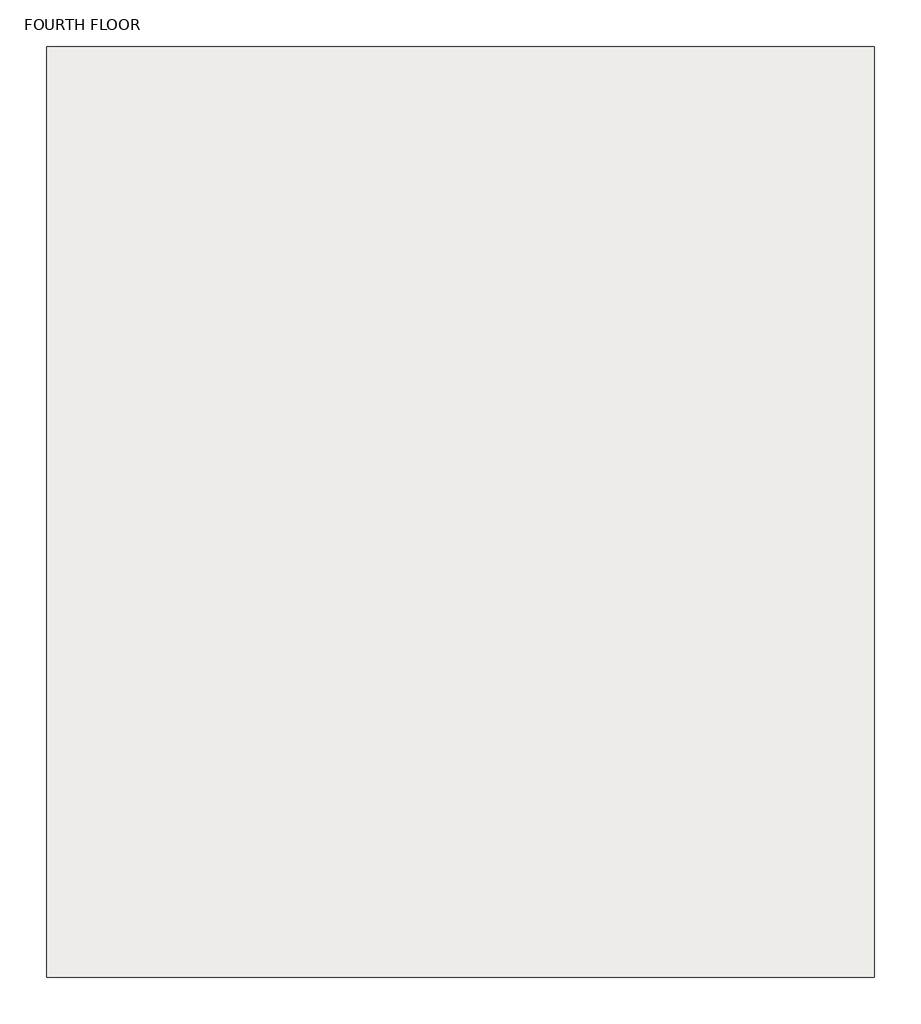
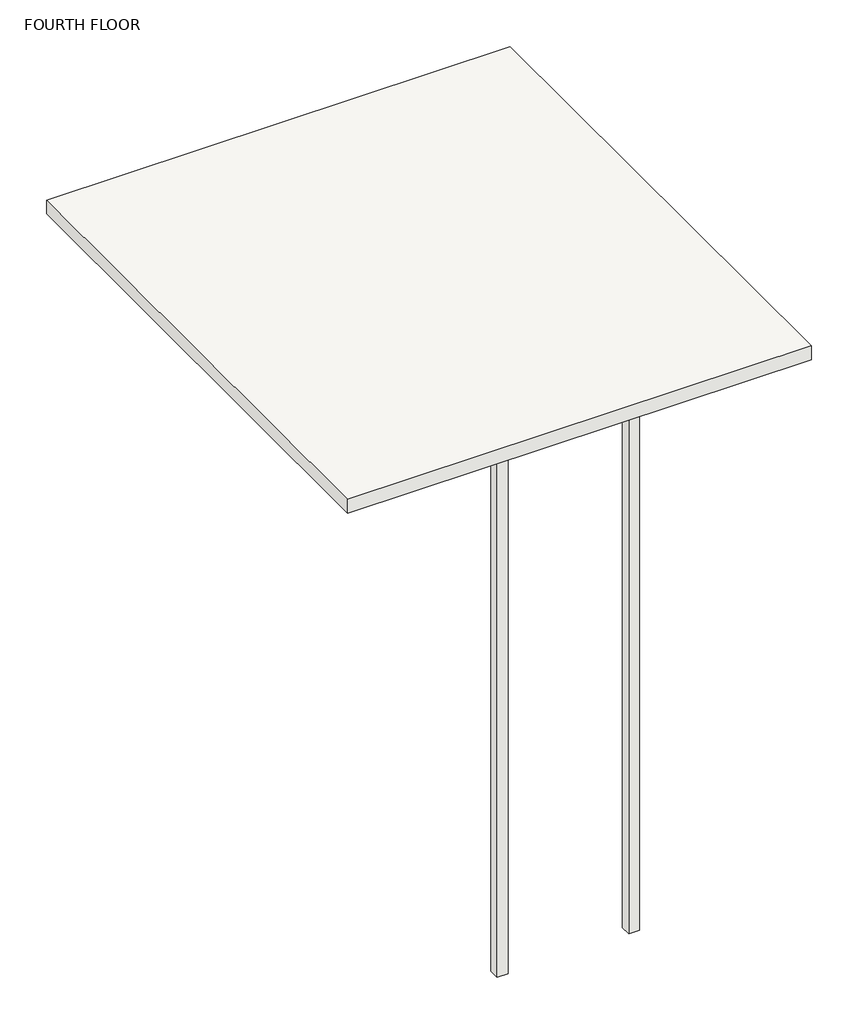
# One storey: 2 slabs.
"""IFC4 building model written with IfcOpenShell, lengths in millimetres."""

from ifc_helpers import new_model, si_unit, frame, origin, place, context, project, spatial, polyline, outline, extrude, transform, mapped, element, save
from components import floors_2_floors_2_8417aeb3

model = new_model("IFC4")

# Units and contexts
model_context = context("Model", 3, world=origin())
ifc_project = project(units=[si_unit("LENGTHUNIT", "METRE", prefix="MILLI")], contexts=[model_context])

# Site, building, storey
site = spatial("IfcSite", under=ifc_project)
building = spatial("IfcBuilding", under=site)
storey = spatial("IfcBuildingStorey", under=building, Name="FOURTH FLOOR", Elevation=12192.0)

# Slabs
placement = place(None, origin())
floors_2_floors_2_shape = floors_2_floors_2_8417aeb3(model_context)
element("IfcSlab", 1, ObjectType="Floors 2 : Floors 2", at=placement, inside=storey, context=model_context, shape_type="MappedRepresentation", body=[
    mapped(floors_2_floors_2_shape, transform((0.0, 0.0, 0.0), x_axis=(1.0, 0.0, 0.0), y_axis=(0.0, 1.0, 0.0), z_axis=(0.0, 0.0, 1.0))),
])
element("IfcSlab", 2, ObjectType="Generic - 12\"", at=placement, inside=storey, context=model_context, shape_type="SweptSolid", body=[
    extrude(outline(polyline([(3431.5769214, -2070.4464178), (-6322.0230786, -2070.4464178), (-6322.0230786, 8902.3535822), (3431.5769214, 8902.3535822), (3431.5769214, -2070.4464178)])), frame((0.0, 0.0, 11887.2), z_axis=(0.0, 0.0, 1.0), x_axis=(1.0, 0.0, 0.0)), (0.0, 0.0, 1.0), 304.8),
])

save(model, "model.ifc")

# Revit data of these elements
# Type "Generic - 12\""
#   Assembly Code = "B1010"
#   Function = 0
#   Layers, outside or top first: 1' - 0" no material (function 1)
# Element 1 (IfcSlab, "Floors 2 : Floors 2")
#   Phase Created = New Construction
#   Materials on its faces: "Default Floor", "1 wood"
# Element 2 (IfcSlab, "Generic - 12\"")
#   Height Offset From Level = 0' - 0"
#   Phase Created = New Construction
#   Materials on its faces: "Default Floor"
# Materials
#   "Default Floor": colour RGB 128 128 128, transparency 0, Cost = 0
#   "1 wood": class "Generic", colour RGB 61 46 37, transparency 0, Cost = 0
